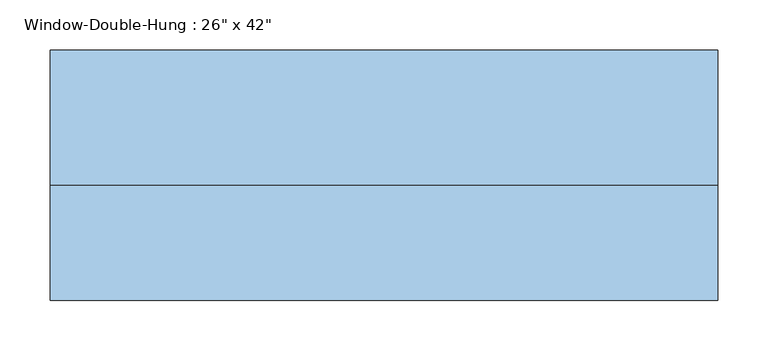
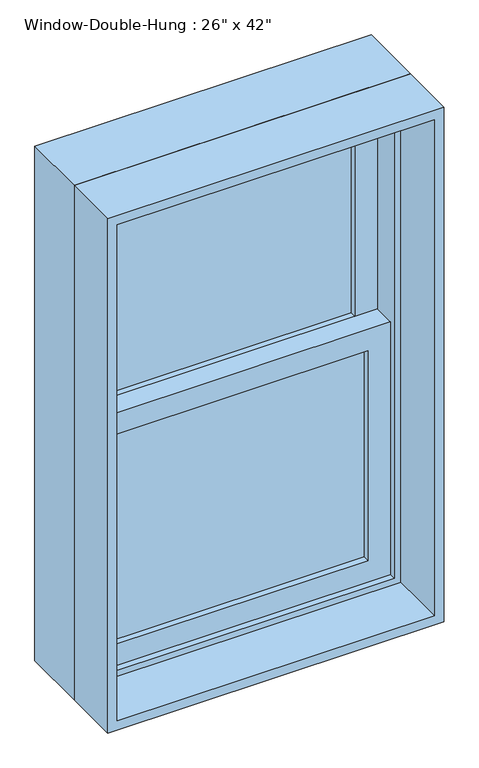
"""IFC4 building model written with IfcOpenShell, lengths in millimetres: window geometry."""

from ifc_helpers import new_model, si_unit, frame, origin, place, context, project, spatial, polyline, outline, extrude, source, transform, mapped, element, save


def window_251dd907(model_context):
    return source(origin(), model_context, "Body", "SweptSolid", [
        extrude(outline(polyline([(254.0, 44.45), (254.0, 38.1), (-254.0, 38.1), (-254.0, 44.45), (254.0, 44.45)])), frame((0.0, 0.0, 990.6), z_axis=(0.0, 0.0, 1.0), x_axis=(1.0, 0.0, 0.0)), (0.0, 0.0, 1.0), 434.975),
        extrude(outline(polyline([(-254.0, 31.75), (254.0, 31.75), (254.0, 25.4), (-254.0, 25.4), (-254.0, 31.75)])), frame((0.0, 0.0, 990.6), z_axis=(0.0, 0.0, 1.0), x_axis=(1.0, 0.0, 0.0)), (0.0, 0.0, 1.0), 434.975),
        extrude(outline(polyline([(254.0, 88.9), (254.0, 82.55), (-254.0, 82.55), (-254.0, 88.9), (254.0, 88.9)])), frame((0.0, 0.0, 1470.025), z_axis=(0.0, 0.0, 1.0), x_axis=(1.0, 0.0, 0.0)), (0.0, 0.0, 1.0), 434.975),
        extrude(outline(polyline([(-254.0, 76.2), (254.0, 76.2), (254.0, 69.85), (-254.0, 69.85), (-254.0, 76.2)])), frame((0.0, 0.0, 1470.025), z_axis=(0.0, 0.0, 1.0), x_axis=(1.0, 0.0, 0.0)), (0.0, 0.0, 1.0), 434.975),
        extrude(outline(polyline([(1470.025, -298.45), (946.15, -298.45), (946.15, 298.45), (1470.025, 298.45), (1470.025, -298.45)]), holes=[polyline([(1425.575, 254.0), (990.6, 254.0), (990.6, -254.0), (1425.575, -254.0), (1425.575, 254.0)])]), frame((0.0, 12.7, 0.0), z_axis=(0.0, 1.0, 0.0), x_axis=(0.0, 0.0, 1.0)), (0.0, 0.0, 1.0), 44.45),
        extrude(outline(polyline([(1949.45, -298.45), (1425.575, -298.45), (1425.575, 298.45), (1949.45, 298.45), (1949.45, -298.45)]), holes=[polyline([(1905.0, 254.0), (1470.025, 254.0), (1470.025, -254.0), (1905.0, -254.0), (1905.0, 254.0)])]), frame((0.0, 57.15, 0.0), z_axis=(0.0, 1.0, 0.0), x_axis=(0.0, 0.0, 1.0)), (0.0, 0.0, 1.0), 44.45),
        extrude(outline(polyline([(1981.2, -330.2), (914.4, -330.2), (914.4, 330.2), (1981.2, 330.2), (1981.2, -330.2)]), holes=[polyline([(1949.45, 298.45), (946.15, 298.45), (946.15, -298.45), (1949.45, -298.45), (1949.45, 298.45)])]), frame((0.0, 0.0, 0.0), z_axis=(0.0, 1.0, 0.0), x_axis=(0.0, 0.0, 1.0)), (0.0, 0.0, 1.0), 133.35),
        extrude(outline(polyline([(1981.2, 330.2), (1981.2, -330.2), (914.4, -330.2), (914.4, 330.2), (1981.2, 330.2)]), holes=[polyline([(1962.15, 311.15), (933.45, 311.15), (933.45, -311.15), (1962.15, -311.15), (1962.15, 311.15)])]), frame((0.0, -114.3, 0.0), z_axis=(0.0, 1.0, 0.0), x_axis=(0.0, 0.0, 1.0)), (0.0, 0.0, 1.0), 114.3),
    ])


if __name__ == "__main__":
    model = new_model("IFC4")
    model_context = context("Model", 3, world=origin())
    ifc_project = project(units=[si_unit("LENGTHUNIT", "METRE", prefix="MILLI")], contexts=[model_context])
    site = spatial("IfcSite", under=ifc_project)
    building = spatial("IfcBuilding", under=site)
    placement = place(None, origin())
    window_shape = window_251dd907(model_context)
    element("IfcWindow", 1, ObjectType="Window-Double-Hung : 26\" x 42\"", at=placement, inside=building, context=model_context, shape_type="MappedRepresentation", body=[
        mapped(window_shape, transform((0.0, 0.0, 0.0), x_axis=(1.0, 0.0, 0.0), y_axis=(0.0, 1.0, 0.0), z_axis=(0.0, 0.0, 1.0))),
    ])
    save(model, "model.ifc")

# Revit data of these elements
# Type "Window-Double-Hung : 26\" x 42\""
#   Type Mark = "11"
#   Fire Rating = "0.5h"
#   Construction Type Id = "DG-DR"
#   Assembly Code = "B2020100"
#   Analytic Construction = "Double glazing - domestic"
#   Wall Thickness [instance default] = 0' - 6"
#   Window Inset [instance default] = 0' - 0"
#   Visual Light Transmittance = 0.81
#   Thermal Resistance (R) = 1.8146 (h·ft²·°F)/BTU
#   Solar Heat Gain Coefficient = 0.76
#   Muntin Width = 1' - 8"
#   Muntin Height = 1' - 5 1/8"
#   Interior Wall Closure [instance default] = 0' - 1 1/2"
#   Rough Width = 2' - 2 1/2"
#   Rough Height = 3' - 6 1/2"
#   Frame Extension [instance default] = 0' - 1 1/4"
#   Exterior Wall Closure [instance default] = 0' - 0 1/2"
#   Extension Jamb [instance default] = 0' - 1 1/2"
#   Heat Transfer Coefficient (U) = 0.5511 BTU/(h·ft²·°F)
#   Height = 3' - 6"
#   Width = 2' - 2"
#   Define Thermal Properties by = 1
#   Top Muntin Visibility = yes
#   Indicator Visibility [instance default] = yes
#   Extension Jamb Visibility [instance default] = yes
#   Interior Trim Visibility [instance default] = yes
#   Exterior Trim Visibility [instance default] = yes
#   Define Thermal Properties by = 1
#   Bottom Muntin Visibility = yes
#   Muntin Pattern = Muntin Pattern_2x2 : Muntin Pattern_2x2
#   Interior Trim Material = Wood - Stained
#   Interior Trim = Trim-Window-Interior-Flat : Picture Frame
#   Exterior Trim Material = Clad - White
#   Exterior Trim = Trim-Window-Exterior-Flat : with Sill
#   Glass Panel Material = Glass
#   Exterior Frame Material = Clad - White
#   Interior Frame Material = Wood - Stained
#   Wall Closure = (empty or 0)
# Element 1 (IfcWindow, "Window-Double-Hung : 26\" x 42\"")
#   Wall Thickness = 0' - 9"
#   Extension Jamb = 0' - 4 1/2"
#   Materials on its faces: "Wood - Stained", "Glass", "Clad - White"
# Materials
#   "Wood - Stained": class "Wood", colour RGB 224 178 126, transparency 0, Cost = 0
#   "Clad - White": class "Wood", colour RGB 242 242 238, transparency 0, Cost = 0
#   "Glass": class "Glass", colour RGB 0 128 192, transparency 0.75, Description = "Soda Lime Glass", Cost = 0
